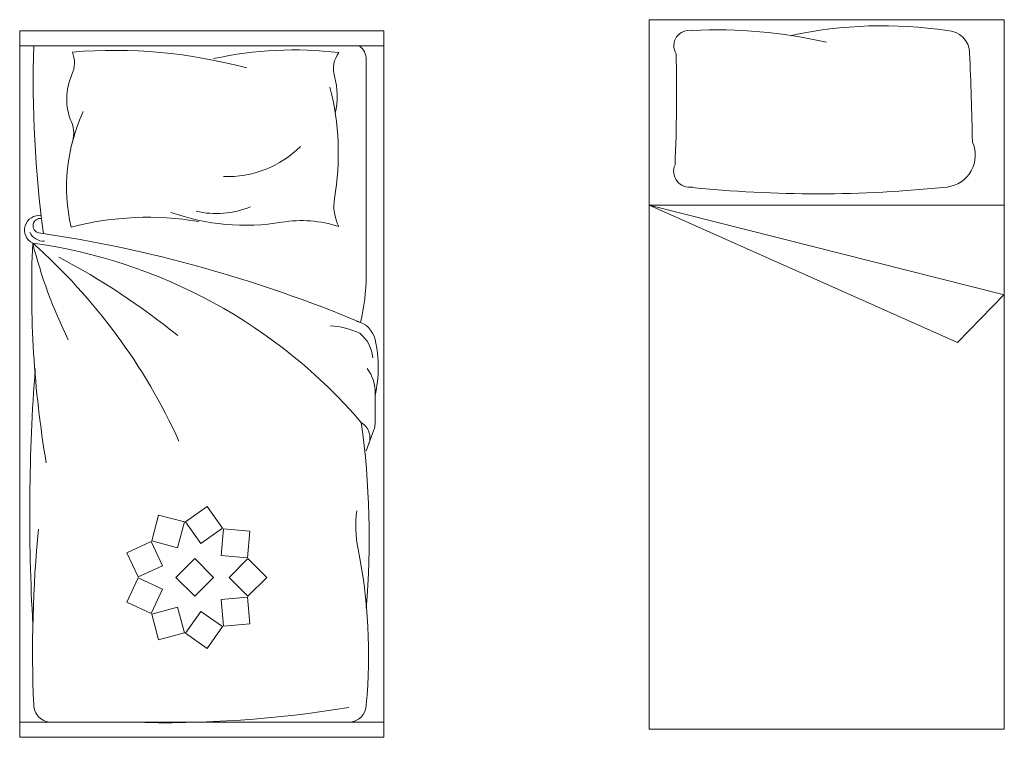
# Model space of a CAD drawing. Units: inches. Extents: x 1994 to 3075, y 3517 to 3950.
# Tile 15 of 58: x 1994.4076 to 1994.5168, y 3553.4715 to 3553.5511. Entities that reach past the tile are written whole.
import ezdxf

# ---------------------------------------------------------------- set-up
doc = ezdxf.new("R2010")
doc.units = ezdxf.units.IN
doc.layers.add('A-FURN-REFR', color=8, linetype='Continuous', lineweight=13)

msp = doc.modelspace()

# ---------------------------------------------------------------- linework, layer by layer
at = {"layer": 'A-FURN-REFR'}
for p, q in [((1994.516758089742, 3553.551120836704), (1994.477388011002, 3553.551120836704)), ((1994.477388011002, 3553.551120836704), (1994.477388011002, 3553.472380679224)), ((1994.516758089742, 3553.472380679224), (1994.516758089742, 3553.551120836704)), ((1994.447944444797, 3553.549896824299), (1994.407559531045, 3553.549896824299)), ((1994.407559531045, 3553.549896824299), (1994.407559531029, 3553.471489836036)), ((1994.447944444797, 3553.549896824299), (1994.447944444781, 3553.471489836036)), ((1994.407559531045, 3553.548223623056), (1994.447944444797, 3553.548223623042)), ((1994.445998861957, 3553.522716254859), (1994.445998861962, 3553.546667156793)), ((1994.477388011002, 3553.53054624855), (1994.511571199707, 3553.515282634939)), ((1994.477388011002, 3553.53054624855), (1994.516768672214, 3553.520607279049)), ((1994.516758089742, 3553.53054624855), (1994.477388011002, 3553.53054624855)), ((1994.511571199707, 3553.515282634939), (1994.516758089742, 3553.520609949874)), ((1994.446971653371, 3553.506268617844), (1994.446971653372, 3553.510086444833)), ((1994.446851447692, 3553.505595349098), (1994.445998861953, 3553.503283804798)), ((1994.428358700177, 3553.497099688378), (1994.425939944141, 3553.495406057169)), ((1994.430052331386, 3553.494680932342), (1994.428358700177, 3553.497099688378)), ((1994.422973943632, 3553.496150210514), (1994.422209714168, 3553.493298067327)), ((1994.42582608682, 3553.495385981051), (1994.422973943632, 3553.496150210514)), ((1994.425061857356, 3553.492533837863), (1994.42582608682, 3553.495385981051)), ((1994.425939944141, 3553.495406057169), (1994.42763357535, 3553.492987301132)), ((1994.42763357535, 3553.492987301132), (1994.430052331386, 3553.494680932342)), ((1994.430152455834, 3553.494623125465), (1994.4298951062, 3553.491681605687)), ((1994.433093975612, 3553.494365775831), (1994.430152455834, 3553.494623125465)), ((1994.432836625978, 3553.491424256054), (1994.433093975612, 3553.494365775831)), ((1994.42213539908, 3553.493209502053), (1994.419459293409, 3553.491961613485)), ((1994.423383287648, 3553.490533396383), (1994.42213539908, 3553.493209502053)), ((1994.422209714168, 3553.493298067327), (1994.425061857356, 3553.492533837863)), ((1994.419459293409, 3553.491961613485), (1994.420707181978, 3553.489285507815)), ((1994.4269706564, 3553.491315614662), (1994.424882742675, 3553.489227700938)), ((1994.429058570124, 3553.489227700938), (1994.4269706564, 3553.491315614662)), ((1994.4298951062, 3553.491681605687), (1994.432836625978, 3553.491424256054)), ((1994.432876168211, 3553.491315614662), (1994.430788254487, 3553.489227700938)), ((1994.434964081935, 3553.489227700938), (1994.432876168211, 3553.491315614662)), ((1994.420707181978, 3553.489285507815), (1994.423383287648, 3553.490533396383)), ((1994.420707181978, 3553.489169894061), (1994.419459293409, 3553.486493788391)), ((1994.423383287648, 3553.487922005493), (1994.420707181978, 3553.489169894061)), ((1994.424882742675, 3553.489227700938), (1994.4269706564, 3553.487139787214)), ((1994.4269706564, 3553.487139787214), (1994.429058570124, 3553.489227700938)), ((1994.430788254487, 3553.489227700938), (1994.432876168211, 3553.487139787214)), ((1994.432876168211, 3553.487139787214), (1994.434964081935, 3553.489227700938)), ((1994.42213539908, 3553.485245899822), (1994.423383287648, 3553.487922005493)), ((1994.419459293409, 3553.486493788391), (1994.42213539908, 3553.485245899822)), ((1994.432836625978, 3553.487031145823), (1994.4298951062, 3553.486773796189)), ((1994.4298951062, 3553.486773796189), (1994.430152455834, 3553.483832276411)), ((1994.433093975612, 3553.484089626046), (1994.432836625978, 3553.487031145823)), ((1994.425061857356, 3553.485921564013), (1994.422209714168, 3553.485157334549)), ((1994.42582608682, 3553.483069420825), (1994.425061857356, 3553.485921564013)), ((1994.42763357535, 3553.485468100745), (1994.425939944141, 3553.483049344708)), ((1994.430052331386, 3553.483774469535), (1994.42763357535, 3553.485468100745)), ((1994.422209714168, 3553.485157334549), (1994.422973943632, 3553.482305191361)), ((1994.428358700177, 3553.481355713498), (1994.430052331386, 3553.483774469535)), ((1994.430152455834, 3553.483832276411), (1994.433093975612, 3553.484089626046)), ((1994.422973943632, 3553.482305191361), (1994.42582608682, 3553.483069420825)), ((1994.425939944141, 3553.483049344708), (1994.428358700177, 3553.481355713498)), ((1994.407559531029, 3553.473163037264), (1994.447944444782, 3553.473163037255)), ((1994.477388011002, 3553.472380679224), (1994.516758089742, 3553.472380679224)), ((1994.407559531045, 3553.471489836036), (1994.447944444781, 3553.471489836036))]:
    msp.add_line(p, q, dxfattribs=at)
for centre, radius, start, end in [((1994.481834909506, 3553.548223112493), 0.0017217387327707, 78.72778623498706, 211.6094986857782), ((1994.481834909506, 3553.548223112493), 0.0017217387327707, 78.72778623498706, 211.6094986857782), ((1994.485024179229, 3553.496351936078), 0.0536356196908511, 77.05638185161688, 93.04883220562752), ((1994.485024179229, 3553.496351936078), 0.0536356196908511, 77.05638185161688, 93.04883220562752), ((1994.503259729437, 3553.502120564467), 0.0483256070365364, 81.47022635647696, 102.1032641982298), ((1994.503259729437, 3553.502120564467), 0.0483256070365364, 81.47022635647696, 102.1032641982298), ((1994.510427544464, 3553.547434054541), 0.0024775836026722, 0, 90), ((1994.510427544464, 3553.547434054541), 0.0024775836026722, 0, 90), ((1994.539632663897, 3553.544510292255), 0.1305694799013457, 178.3703169121375, 187.5322278354393), ((1994.410428549245, 3553.54634209869), 0.0032028341489732, 335.7877323280015, 21.71237864400314), ((1994.418016480052, 3553.491209131769), 0.0565064023996118, 74.89247536308716, 94.681970907379), ((1994.437996176823, 3553.506299895526), 0.0414680575843914, 83.14136388124066, 102.4247502365447), ((1994.444053279126, 3553.546667156793), 0.0019455828353276, 359.9999999880876, 53.13010234330246), ((1994.445474346734, 3553.54566130914), 0.0031075126812102, 144.3787648229011, 195.1987658355305), ((1994.303043380688, 3553.542975349651), 0.1773784605747312, 357.4333292641344, 1.403751564921032), ((1994.303043380688, 3553.542975349651), 0.1773784605747312, 357.4333292641344, 1.403751564921032), ((1994.218212895161, 3553.532845571028), 0.2950531070603349, 0.9125644663952034, 2.834064295864955), ((1994.218212895161, 3553.532845571028), 0.2950531070603349, 0.9125644663952034, 2.834064295864955), ((1994.41934758867, 3553.542331427842), 0.0065764677133891, 155.7877323280015, 202.8808293159797), ((1994.434179928862, 3553.542592944963), 0.0085962787467616, 347.311957921453, 15.19876583553051), ((1994.413040326413, 3553.536279099003), 0.0298558147000044, 350.3711224665587, 14.25995084780135), ((1994.432614730474, 3553.532568198205), 0.0198519972069101, 155.1179531461462, 192.9861889591517), ((1994.410211220381, 3553.538475676689), 0.0033401870886801, 339.0160855821216, 22.88082931597971), ((1994.430608653737, 3553.545159879192), 0.0114567055564695, 267.8294752673963, 315.0098308273483), ((1994.509993806796, 3553.536079145155), 0.0035513056944607, 277.015318444972, 24.37436785420747), ((1994.509993806796, 3553.536079145155), 0.0035513056944607, 277.015318444972, 24.37436785420747), ((1994.481872617974, 3553.534310544359), 0.0017813637547286, 156.1084115545774, 279.6575795622506), ((1994.481872617974, 3553.534310544359), 0.0017813637547286, 156.1084115545774, 279.6575795622506), ((1994.49602869432, 3553.669840813299), 0.1380394109326758, 264.1139139330622, 275.9873971424126), ((1994.49602869432, 3553.669840813299), 0.1380394109326758, 264.1139139330622, 275.9873971424126), ((1994.447401230944, 3553.530449571898), 0.004996088352876, 170.3711224665586, 206.9649370961853), ((1994.429344930729, 3553.539599281242), 0.009989213432703, 257.148031947205, 292.3825063085086), ((1994.409709156654, 3553.527774762038), 0.0016105685091622, 81.6091039781453, 243.938180591863), ((1994.409856404249, 3553.528265221731), 0.0008128892221172, 81.29146871137522, 258.1255955891823), ((1994.421762975311, 3553.495497603466), 0.0336972432594088, 80.32657587842615, 104.5973118255227), ((1994.432603125125, 3553.552948825775), 0.0246390736856652, 250.3559327023518, 279.3925899659531), ((1994.438837828029, 3553.515257787318), 0.0135641447689492, 72.35976010254194, 99.39258996595309), ((1994.410177159693, 3553.528161241527), 0.0016095821071006, 202.6051908922757, 274.4988817166678), ((1994.387903594146, 3553.380291995377), 0.1487813656996577, 67.27623853958569, 81.58010286503209), ((1994.525518351333, 3553.521228643783), 0.1166283141987217, 177.4940716817132, 189.5094068679036), ((1994.36553118723, 3553.477274337105), 0.065543355857517, 24.38326925012849, 48.45324971012612), ((1994.400976268203, 3553.468323236192), 0.0585572615340703, 40.58068443299209, 82.12279458076166), ((1994.461440699485, 3553.539586758712), 0.0540893550839264, 194.1893851607317, 206.3095844034524), ((1994.373550138829, 3553.452348197666), 0.0819509525067612, 51.03759283326017, 62.08562985249065), ((1994.421281565468, 3553.523047893384), 0.0247195212287987, 347.0890423172248, 359.2312934508153), ((1994.441436376705, 3553.508040224145), 0.0091331594194461, 65.03385580996276, 86.4640048798947), ((1994.444326624697, 3553.515011147364), 0.0027238159694586, 12.88269036848606, 78.38686031445394), ((1994.4427893855, 3553.513274218948), 0.0039416012902181, 4.684898432501862, 50.59840531545589), ((1994.433501769207, 3553.512535366099), 0.013828183994568, 346.9286456497866, 12.88269036848606), ((1994.625487184805, 3553.496154656567), 0.2168115609509192, 175.697202442643, 183.2229785434103), ((1994.442784465351, 3553.509837803962), 0.0041945638393764, 356.601689895136, 37.73019638534235), ((1994.353150230714, 3553.493646793476), 0.0931787946855045, 355.1752823324409, 7.876466900264919), ((1994.44446212916, 3553.504739650832), 0.0019455828353278, 339.7541012352643, 59.48721857724742), ((1994.445026070535, 3553.506268617845), 0.0019455828353276, 339.7541012352643, 359.9999999880876), ((1994.445026070535, 3553.506268617845), 0.0019455828353276, 339.7541012352643, 359.9999999880876), ((1994.457818004923, 3553.494933181291), 0.0129749866847535, 172.4746658505032, 191.3425348756069), ((1994.550279032558, 3553.481090515266), 0.1412897221787423, 174.5126540947314, 182.4265021931356), ((1994.386719837595, 3553.480671468557), 0.0595394659951302, 354.6389628949611, 11.34253487560691), ((1994.411061580134, 3553.475108620109), 0.0019455828353276, 179.9999999880876, 269.9999999880876), ((1994.423604056635, 3553.597248944618), 0.1241401229318277, 268.3066004926072, 279.4831521227457), ((1994.444053279111, 3553.47510862011), 0.0019455828353276, 269.9999999880876, 359.9999999880876)]:
    msp.add_arc(centre, radius, start, end, dxfattribs=at)

doc.saveas('drawing.dxf')
